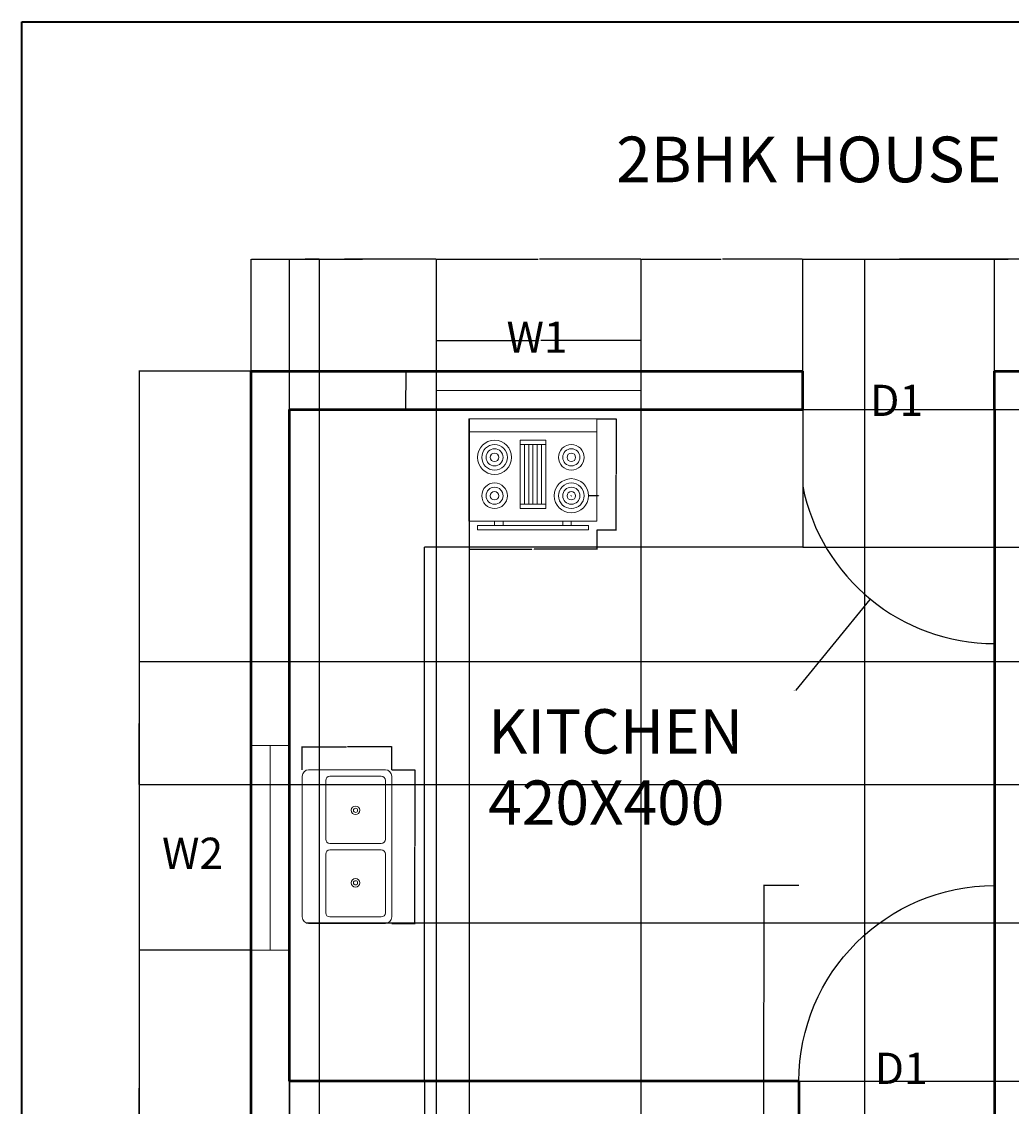
# Model space of a CAD drawing. Units: centimetres. Extents: x 2050 to 3144, y 831 to 2296.
# Tile 6 of 7: x 2050 to 2640, y 1650 to 2296. Entities that reach past the tile are written whole.
import ezdxf

# ---------------------------------------------------------------- set-up
doc = ezdxf.new("R2010")
doc.units = ezdxf.units.CM
for name, color, linetype, lineweight in [('A-ANNO-DIMS', 2, 'Continuous', 18), ('A-ANNO-TEXT', 7, 'Continuous', 18), ('A-ANNO-TTLB', 7, 'Continuous', 35), ('A-AREA-IDEN', 7, 'Continuous', 25), ('A-DOOR', 3, 'Continuous', 25), ('A-EQPM', 9, 'Continuous', 18), ('A-FLOR-CASE', 8, 'Continuous', 25), ('A-FLOR-FIXT', 8, 'Continuous', 18), ('A-GLAZ', 4, 'Continuous', 18), ('A-WALL', 7, 'Continuous', 50)]:
    doc.layers.add(name, color=color, linetype=linetype, lineweight=lineweight)
doc.styles.get("Standard").update_dxf_attribs({"font": 'arial.ttf'})
doc.dimstyles.get("Standard").update_dxf_attribs({"dimtxt": 0.18, "dimasz": 0.18, "dimexe": 0.18, "dimexo": 0.0625, "dimgap": 0.09, "dimtad": 0, "dimtih": 1, "dimtoh": 1, "dimdec": 4, "dimzin": 0, "dimdsep": 46, "dimtxsty": 'Standard', "dimcen": 0.09, "dimadec": 0, "dimazin": 0, "dimtfac": 1, "dimtdec": 4, "dimtofl": 0, "dimtmove": 0, "dimatfit": 3, "dimfxl": 1, "dimtolj": 1, "dimtzin": 0, "dimarcsym": 0})

# ---------------------------------------------------------------- blocks, each defined once
blk = doc.blocks.new('Sink-double - 36 in top')
for p, q in [((-18, -4), (18, -4)), ((-0.75, -18.5), (-0.75, -6.5)), ((0.75, -6.5), (0.75, -18.5))]:
    blk.add_line(p, q)
for points in [[(-16.5, 0), (16.5, 0)], [(-18, -19.5), (-18, -1.5)], [(18, -1.5), (18, -19.5)], [(-16.5, -18.5), (-16.5, -6.5)], [(-15.5, -5.5), (-1.75, -5.5)], [(1.75, -5.5), (15.5, -5.5)], [(16.5, -6.5), (16.5, -18.5)], [(-1.75, -19.5), (-15.5, -19.5)], [(15.5, -19.5), (1.75, -19.5)], [(16.5, -21), (-16.5, -21)]]:
    blk.add_lwpolyline(points)
for centre, radius in [((-8.5, -12.5), 1), ((-8.5, -12.5), 0.5), ((8.5, -12.5), 1), ((8.5, -12.5), 0.5)]:
    blk.add_circle(centre, radius)
for centre, radius, start, end in [((-16.5, -1.5), 1.5, 90, 180), ((16.5, -1.5), 1.5, 0, 90), ((-15.5, -6.5), 1, 90, 180), ((-1.75, -6.5), 1, 0, 90), ((1.75, -6.5), 1, 90, 180), ((15.5, -6.5), 1, 0, 90), ((-16.5, -19.5), 1.5, 180, 270), ((-15.5, -18.5), 1, 180, 270), ((-1.75, -18.5), 1, 270, 0), ((1.75, -18.5), 1, 180, 270), ((15.5, -18.5), 1, 270, 0), ((16.5, -19.5), 1.5, 270, 0)]:
    blk.add_arc(centre, radius, start, end)
blk = doc.blocks.new('Range-Oven - 30 in top')
for p, q in [((0, -3), (30, -3)), ((12, -6), (18, -6)), ((13, -20), (13, -6)), ((14, -6), (14, -20)), ((15, -20), (15, -6)), ((16, -6), (16, -20)), ((17, -20), (17, -6)), ((18, -20), (12, -20)), ((6, -24), (6, -25)), ((8, -25), (8, -24)), ((22, -25), (22, -24)), ((24, -24), (24, -25))]:
    blk.add_line(p, q)
for points in [[(0, -24), (0, 0), (30, 0), (30, -24)], [(12, -21), (12, -5), (18, -5), (18, -21)], [(2, -26), (2, -25), (28, -25), (28, -26)]]:
    blk.add_lwpolyline(points, close=True)
for centre, radius in [((6, -9), 4), ((6, -9), 3), ((6, -9), 2), ((24, -9), 3), ((24, -9), 2), ((6, -9), 1), ((24, -9), 1), ((6, -18), 3), ((24, -18), 4), ((24, -18), 3), ((6, -18), 2), ((6, -18), 1), ((24, -18), 2), ((24, -18), 1)]:
    blk.add_circle(centre, radius)
blk = doc.blocks.new('DOOR-D1-1165')
blk.add_line((116.51, 0), (116.51, 139.37))
blk.add_arc((116.51, 116.51), 116.51, 180, 270)
blk = doc.blocks.new('WIN-1219')
for p, q in [((0, 22.86), (0, 0)), ((121.92, 22.86), (121.92, 0)), ((0, 11.43), (121.92, 11.43))]:
    blk.add_line(p, q)
blk = doc.blocks.new('*D15')
at = {"layer": 'A-ANNO-DIMS', "color": 0, "lineweight": -2, "transparency": 16777216}
for p, q in [((2513.3, 1781.4), (2492.28, 1781.4)), ((2492.46, 1781.22), (2492.46, 1711.9)), ((2492.46, 1642.21), (2492.46, 1711.53)), ((2513.3, 1642.03), (2492.28, 1642.03))]:
    blk.add_line(p, q, dxfattribs=at)
at = {"layer": 'A-ANNO-DIMS', "color": 0, "transparency": 16777216}
for points in [[(2492.43, 1781.22), (2492.49, 1781.22), (2492.46, 1781.4)], [(2492.43, 1642.21), (2492.49, 1642.21), (2492.46, 1642.03)]]:
    blk.add_solid(points, dxfattribs=at)
at = {"layer": 'Defpoints', "color": 0, "transparency": 16777216}
for p in [(2513.36, 1781.4), (2492.46, 1642.03), (2513.36, 1642.03)]:
    blk.add_point(p, dxfattribs=at)
at = {"layer": 'A-ANNO-DIMS', "color": 0, "transparency": 16777216, "insert": (2492.46, 1711.72), "char_height": 0.18, "attachment_point": 5}
blk.add_mtext('\\A1;DOOR D1 139 TYP.', dxfattribs=at)
blk = doc.blocks.new('*D17')
at = {"layer": 'A-ANNO-DIMS', "color": 0, "lineweight": -2, "transparency": 16777216}
for p, q in [((2297.47, 2087.82), (2297.47, 2106.22)), ((2297.65, 2106.04), (2357.25, 2106.04)), ((2419.21, 2106.04), (2359.62, 2106.04)), ((2419.39, 2087.82), (2419.39, 2106.22))]:
    blk.add_line(p, q, dxfattribs=at)
at = {"layer": 'A-ANNO-DIMS', "color": 0, "transparency": 16777216}
for points in [[(2297.65, 2106.07), (2297.65, 2106.01), (2297.47, 2106.04)], [(2419.21, 2106.07), (2419.21, 2106.01), (2419.39, 2106.04)]]:
    blk.add_solid(points, dxfattribs=at)
at = {"layer": 'Defpoints', "color": 0, "transparency": 16777216}
for p in [(2419.39, 2106.04), (2297.47, 2087.75), (2419.39, 2087.75)]:
    blk.add_point(p, dxfattribs=at)
at = {"layer": 'A-ANNO-DIMS', "color": 0, "transparency": 16777216, "insert": (2358.43, 2106.04), "char_height": 0.18, "attachment_point": 5}
blk.add_mtext('\\A1;WINDOW 122 TYP.', dxfattribs=at)
blk = doc.blocks.new('*D18')
at = {"layer": 'A-ANNO-DIMS', "color": 0, "lineweight": -2, "transparency": 16777216}
for p, q in [((2297.41, 2087.75), (2279.01, 2087.75)), ((2279.19, 2087.57), (2279.19, 2076.51)), ((2279.19, 2065.07), (2279.19, 2076.14)), ((2297.41, 2064.89), (2279.01, 2064.89))]:
    blk.add_line(p, q, dxfattribs=at)
at = {"layer": 'A-ANNO-DIMS', "color": 0, "transparency": 16777216}
for points in [[(2279.16, 2087.57), (2279.22, 2087.57), (2279.19, 2087.75)], [(2279.16, 2065.07), (2279.22, 2065.07), (2279.19, 2064.89)]]:
    blk.add_solid(points, dxfattribs=at)
at = {"layer": 'Defpoints', "color": 0, "transparency": 16777216}
for p in [(2279.19, 2087.75), (2297.47, 2087.75), (2297.47, 2064.89)]:
    blk.add_point(p, dxfattribs=at)
at = {"layer": 'A-ANNO-DIMS', "color": 0, "transparency": 16777216, "insert": (2279.19, 2076.32), "char_height": 0.18, "attachment_point": 5}
blk.add_mtext('\\A1;23 TYP.', dxfattribs=at)
blk = doc.blocks.new('*D25')
at = {"layer": 'A-ANNO-DIMS', "color": 0, "lineweight": -2, "transparency": 16777216}
for p, q in [((2270.89, 1850.36), (2284.72, 1850.36)), ((2284.54, 1850.18), (2284.54, 1804.83)), ((2284.54, 1759.1), (2284.54, 1804.46)), ((2270.89, 1758.92), (2284.72, 1758.92))]:
    blk.add_line(p, q, dxfattribs=at)
at = {"layer": 'A-ANNO-DIMS', "color": 0, "transparency": 16777216}
for points in [[(2284.51, 1850.18), (2284.57, 1850.18), (2284.54, 1850.36)], [(2284.51, 1759.1), (2284.57, 1759.1), (2284.54, 1758.92)]]:
    blk.add_solid(points, dxfattribs=at)
at = {"layer": 'Defpoints', "color": 0, "transparency": 16777216}
for p in [(2270.83, 1850.36), (2284.54, 1850.36), (2270.83, 1758.92)]:
    blk.add_point(p, dxfattribs=at)
at = {"layer": 'A-ANNO-DIMS', "color": 0, "transparency": 16777216, "insert": (2284.54, 1804.64), "char_height": 0.18, "attachment_point": 5}
blk.add_mtext('\\A1;SINK 91', dxfattribs=at)
blk = doc.blocks.new('*D26')
at = {"layer": 'A-ANNO-DIMS', "color": 0, "lineweight": -2, "transparency": 16777216}
for p, q in [((2217.49, 1850.42), (2217.49, 1864.26)), ((2217.67, 1864.08), (2243.94, 1864.08)), ((2270.65, 1864.08), (2244.38, 1864.08)), ((2270.83, 1850.42), (2270.83, 1864.26))]:
    blk.add_line(p, q, dxfattribs=at)
at = {"layer": 'A-ANNO-DIMS', "color": 0, "transparency": 16777216}
for points in [[(2217.67, 1864.11), (2217.67, 1864.05), (2217.49, 1864.08)], [(2270.65, 1864.11), (2270.65, 1864.05), (2270.83, 1864.08)]]:
    blk.add_solid(points, dxfattribs=at)
at = {"layer": 'Defpoints', "color": 0, "transparency": 16777216}
for p in [(2217.49, 1864.08), (2217.49, 1850.36), (2270.83, 1850.36)]:
    blk.add_point(p, dxfattribs=at)
at = {"layer": 'A-ANNO-DIMS', "color": 0, "transparency": 16777216, "insert": (2244.16, 1864.08), "char_height": 0.18, "attachment_point": 5}
blk.add_mtext('\\A1;53', dxfattribs=at)
blk = doc.blocks.new('*D27')
at = {"layer": 'A-ANNO-DIMS', "color": 0, "lineweight": -2, "transparency": 16777216}
for p, q in [((2316.84, 1993.19), (2316.84, 1981.64)), ((2393.04, 1993.19), (2393.04, 1981.64)), ((2317.02, 1981.82), (2354.24, 1981.82)), ((2392.86, 1981.82), (2355.63, 1981.82))]:
    blk.add_line(p, q, dxfattribs=at)
at = {"layer": 'A-ANNO-DIMS', "color": 0, "transparency": 16777216}
for points in [[(2317.02, 1981.85), (2317.02, 1981.79), (2316.84, 1981.82)], [(2392.86, 1981.85), (2392.86, 1981.79), (2393.04, 1981.82)]]:
    blk.add_solid(points, dxfattribs=at)
at = {"layer": 'Defpoints', "color": 0, "transparency": 16777216}
for p in [(2316.84, 1993.25), (2393.04, 1993.25), (2393.04, 1981.82)]:
    blk.add_point(p, dxfattribs=at)
at = {"layer": 'A-ANNO-DIMS', "color": 0, "transparency": 16777216, "insert": (2354.94, 1981.82), "char_height": 0.18, "attachment_point": 5}
blk.add_mtext('\\A1;RANGE 76', dxfattribs=at)
blk = doc.blocks.new('*D28')
at = {"layer": 'A-ANNO-DIMS', "color": 0, "lineweight": -2, "transparency": 16777216}
for p, q in [((2393.1, 2059.29), (2404.65, 2059.29)), ((2404.47, 2059.11), (2404.47, 2026.45)), ((2404.47, 1993.43), (2404.47, 2026.09)), ((2393.1, 1993.25), (2404.65, 1993.25))]:
    blk.add_line(p, q, dxfattribs=at)
at = {"layer": 'A-ANNO-DIMS', "color": 0, "transparency": 16777216}
for points in [[(2404.44, 2059.11), (2404.5, 2059.11), (2404.47, 2059.29)], [(2404.44, 1993.43), (2404.5, 1993.43), (2404.47, 1993.25)]]:
    blk.add_solid(points, dxfattribs=at)
at = {"layer": 'Defpoints', "color": 0, "transparency": 16777216}
for p in [(2393.04, 2059.29), (2404.47, 2059.29), (2393.04, 1993.25)]:
    blk.add_point(p, dxfattribs=at)
at = {"layer": 'A-ANNO-DIMS', "color": 0, "transparency": 16777216, "insert": (2404.47, 2026.27), "char_height": 0.18, "attachment_point": 5}
blk.add_mtext('\\A1;66', dxfattribs=at)
blk = doc.blocks.new('*D32')
at = {"layer": 'A-ANNO-DIMS', "color": 0, "lineweight": -2, "transparency": 16777216}
for p, q in [((2186.94, 2087.75), (2120.23, 2087.75)), ((2120.41, 2087.57), (2120.41, 1582.22)), ((2120.41, 1076.49), (2120.41, 1581.85)), ((2186.94, 1076.31), (2120.23, 1076.31))]:
    blk.add_line(p, q, dxfattribs=at)
at = {"layer": 'A-ANNO-DIMS', "color": 0, "transparency": 16777216}
for points in [[(2120.38, 2087.57), (2120.44, 2087.57), (2120.41, 2087.75)], [(2120.38, 1076.49), (2120.44, 1076.49), (2120.41, 1076.31)]]:
    blk.add_solid(points, dxfattribs=at)
at = {"layer": 'Defpoints', "color": 0, "transparency": 16777216}
for p in [(2120.41, 2087.75), (2187.01, 2087.75), (2187.01, 1076.31)]:
    blk.add_point(p, dxfattribs=at)
at = {"layer": 'A-ANNO-DIMS', "color": 0, "transparency": 16777216, "insert": (2120.41, 1582.03), "char_height": 0.18, "attachment_point": 5}
blk.add_mtext('\\A1;1011.4', dxfattribs=at)
blk = doc.blocks.new('*D33')
at = {"layer": 'A-ANNO-DIMS', "color": 0, "lineweight": -2, "transparency": 16777216}
for p, q in [((2187.01, 2087.82), (2187.01, 2154.53)), ((2187.19, 2154.35), (2241.78, 2154.35)), ((2297.29, 2154.35), (2242.7, 2154.35)), ((2297.47, 2087.82), (2297.47, 2154.53))]:
    blk.add_line(p, q, dxfattribs=at)
at = {"layer": 'A-ANNO-DIMS', "color": 0, "transparency": 16777216}
for points in [[(2187.19, 2154.38), (2187.19, 2154.32), (2187.01, 2154.35)], [(2297.29, 2154.38), (2297.29, 2154.32), (2297.47, 2154.35)]]:
    blk.add_solid(points, dxfattribs=at)
at = {"layer": 'Defpoints', "color": 0, "transparency": 16777216}
for p in [(2297.47, 2154.35), (2187.01, 2087.75), (2297.47, 2087.75)]:
    blk.add_point(p, dxfattribs=at)
at = {"layer": 'A-ANNO-DIMS', "color": 0, "transparency": 16777216, "insert": (2242.24, 2154.35), "char_height": 0.18, "attachment_point": 5}
blk.add_mtext('\\A1;110.47', dxfattribs=at)
blk = doc.blocks.new('*D34')
at = {"layer": 'A-ANNO-DIMS', "color": 0, "lineweight": -2, "transparency": 16777216}
for p, q in [((2419.39, 2087.82), (2419.39, 2154.53)), ((2419.57, 2154.35), (2467.12, 2154.35)), ((2515.45, 2154.35), (2467.9, 2154.35)), ((2515.63, 2087.82), (2515.63, 2154.53))]:
    blk.add_line(p, q, dxfattribs=at)
at = {"layer": 'A-ANNO-DIMS', "color": 0, "transparency": 16777216}
for points in [[(2419.57, 2154.38), (2419.57, 2154.32), (2419.39, 2154.35)], [(2515.45, 2154.38), (2515.45, 2154.32), (2515.63, 2154.35)]]:
    blk.add_solid(points, dxfattribs=at)
at = {"layer": 'Defpoints', "color": 0, "transparency": 16777216}
for p in [(2515.63, 2154.35), (2419.39, 2087.75), (2515.63, 2087.75)]:
    blk.add_point(p, dxfattribs=at)
at = {"layer": 'A-ANNO-DIMS', "color": 0, "transparency": 16777216, "insert": (2467.51, 2154.35), "char_height": 0.18, "attachment_point": 5}
blk.add_mtext('\\A1;96.23', dxfattribs=at)
blk = doc.blocks.new('*D35')
at = {"layer": 'A-ANNO-DIMS', "color": 0, "lineweight": -2, "transparency": 16777216}
for p, q in [((2515.63, 2087.82), (2515.63, 2154.53)), ((2515.81, 2154.35), (2572.29, 2154.35)), ((2629.69, 2154.35), (2573.2, 2154.35)), ((2629.87, 2087.82), (2629.87, 2154.53))]:
    blk.add_line(p, q, dxfattribs=at)
at = {"layer": 'A-ANNO-DIMS', "color": 0, "transparency": 16777216}
for points in [[(2515.81, 2154.38), (2515.81, 2154.32), (2515.63, 2154.35)], [(2629.69, 2154.38), (2629.69, 2154.32), (2629.87, 2154.35)]]:
    blk.add_solid(points, dxfattribs=at)
at = {"layer": 'Defpoints', "color": 0, "transparency": 16777216}
for p in [(2629.87, 2154.35), (2515.63, 2087.75), (2629.87, 2087.75)]:
    blk.add_point(p, dxfattribs=at)
at = {"layer": 'A-ANNO-DIMS', "color": 0, "transparency": 16777216, "insert": (2572.75, 2154.35), "char_height": 0.18, "attachment_point": 5}
blk.add_mtext('\\A1;114.24', dxfattribs=at)
blk = doc.blocks.new('*D42')
at = {"layer": 'A-ANNO-DIMS', "color": 0, "lineweight": -2, "transparency": 16777216}
for p, q in [((2186.94, 1742.97), (2120.23, 1742.97)), ((2120.41, 1742.79), (2120.41, 1661.12)), ((2120.41, 1579.07), (2120.41, 1660.75)), ((2186.94, 1578.89), (2120.23, 1578.89))]:
    blk.add_line(p, q, dxfattribs=at)
at = {"layer": 'A-ANNO-DIMS', "color": 0, "transparency": 16777216}
for points in [[(2120.38, 1742.79), (2120.44, 1742.79), (2120.41, 1742.97)], [(2120.38, 1579.07), (2120.44, 1579.07), (2120.41, 1578.89)]]:
    blk.add_solid(points, dxfattribs=at)
at = {"layer": 'Defpoints', "color": 0, "transparency": 16777216}
for p in [(2120.41, 1742.97), (2187.01, 1742.97), (2187.01, 1578.89)]:
    blk.add_point(p, dxfattribs=at)
at = {"layer": 'A-ANNO-DIMS', "color": 0, "transparency": 16777216, "insert": (2120.41, 1660.93), "char_height": 0.18, "attachment_point": 5}
blk.add_mtext('\\A1;164.08', dxfattribs=at)
blk = doc.blocks.new('*D47')
at = {"layer": 'A-ANNO-DIMS', "color": 0, "lineweight": -2, "transparency": 16777216}
for p, q in [((2209.87, 1099.24), (2209.87, 2154.53)), ((2210.05, 2154.35), (2253.35, 2154.35)), ((2297.29, 2154.35), (2253.99, 2154.35)), ((2297.47, 1099.24), (2297.47, 2154.53))]:
    blk.add_line(p, q, dxfattribs=at)
at = {"layer": 'A-ANNO-DIMS', "color": 0, "transparency": 16777216}
for points in [[(2210.05, 2154.38), (2210.05, 2154.32), (2209.87, 2154.35)], [(2297.29, 2154.38), (2297.29, 2154.32), (2297.47, 2154.35)]]:
    blk.add_solid(points, dxfattribs=at)
at = {"layer": 'Defpoints', "color": 0, "transparency": 16777216}
for p in [(2297.47, 2154.35), (2209.87, 1099.17), (2297.47, 1099.17)]:
    blk.add_point(p, dxfattribs=at)
at = {"layer": 'A-ANNO-DIMS', "color": 0, "transparency": 16777216, "insert": (2253.67, 2154.35), "char_height": 0.18, "attachment_point": 5}
blk.add_mtext('\\A1;87.6', dxfattribs=at)
blk = doc.blocks.new('*D48')
at = {"layer": 'A-ANNO-DIMS', "color": 0, "lineweight": -2, "transparency": 16777216}
for p, q in [((2552.73, 1211.94), (2552.73, 2154.53)), ((2552.91, 2154.35), (2610.59, 2154.35)), ((2669.05, 2154.35), (2611.37, 2154.35)), ((2669.23, 1211.94), (2669.23, 2154.53))]:
    blk.add_line(p, q, dxfattribs=at)
at = {"layer": 'A-ANNO-DIMS', "color": 0, "transparency": 16777216}
for points in [[(2552.91, 2154.38), (2552.91, 2154.32), (2552.73, 2154.35)], [(2669.05, 2154.38), (2669.05, 2154.32), (2669.23, 2154.35)]]:
    blk.add_solid(points, dxfattribs=at)
at = {"layer": 'Defpoints', "color": 0, "transparency": 16777216}
for p in [(2669.23, 2154.35), (2552.73, 1211.87), (2669.23, 1211.87)]:
    blk.add_point(p, dxfattribs=at)
at = {"layer": 'A-ANNO-DIMS', "color": 0, "transparency": 16777216, "insert": (2610.98, 2154.35), "char_height": 0.18, "attachment_point": 5}
blk.add_mtext('\\A1;116.5', dxfattribs=at)
blk = doc.blocks.new('*D53')
at = {"layer": 'A-ANNO-DIMS', "color": 0, "lineweight": -2, "transparency": 16777216}
for p, q in [((2209.87, 1664.83), (2209.87, 1009.53)), ((2290.25, 1664.83), (2290.25, 1009.53)), ((2210.05, 1009.71), (2249.67, 1009.71)), ((2290.07, 1009.71), (2250.45, 1009.71))]:
    blk.add_line(p, q, dxfattribs=at)
at = {"layer": 'A-ANNO-DIMS', "color": 0, "transparency": 16777216}
for points in [[(2210.05, 1009.74), (2210.05, 1009.68), (2209.87, 1009.71)], [(2290.07, 1009.74), (2290.07, 1009.68), (2290.25, 1009.71)]]:
    blk.add_solid(points, dxfattribs=at)
at = {"layer": 'Defpoints', "color": 0, "transparency": 16777216}
for p in [(2209.87, 1664.89), (2290.25, 1664.89), (2290.25, 1009.71)]:
    blk.add_point(p, dxfattribs=at)
at = {"layer": 'A-ANNO-DIMS', "color": 0, "transparency": 16777216, "insert": (2250.06, 1009.71), "char_height": 0.18, "attachment_point": 5}
blk.add_mtext('\\A1;80.39', dxfattribs=at)
blk = doc.blocks.new('*D54')
at = {"layer": 'A-ANNO-DIMS', "color": 0, "lineweight": -2, "transparency": 16777216}
for p, q in [((2515.69, 2064.89), (3042.37, 2064.89)), ((3042.19, 2064.71), (3042.19, 2024.09)), ((3042.19, 1983.1), (3042.19, 2023.73)), ((2515.69, 1982.92), (3042.37, 1982.92))]:
    blk.add_line(p, q, dxfattribs=at)
at = {"layer": 'A-ANNO-DIMS', "color": 0, "transparency": 16777216}
for points in [[(3042.16, 2064.71), (3042.22, 2064.71), (3042.19, 2064.89)], [(3042.16, 1983.1), (3042.22, 1983.1), (3042.19, 1982.92)]]:
    blk.add_solid(points, dxfattribs=at)
at = {"layer": 'Defpoints', "color": 0, "transparency": 16777216}
for p in [(2515.63, 2064.89), (3042.19, 2064.89), (2515.63, 1982.92)]:
    blk.add_point(p, dxfattribs=at)
at = {"layer": 'A-ANNO-DIMS', "color": 0, "transparency": 16777216, "insert": (3042.19, 2023.91), "char_height": 0.18, "attachment_point": 5}
blk.add_mtext('\\A1;81.97', dxfattribs=at)
blk = doc.blocks.new('*D61')
at = {"layer": 'A-ANNO-DIMS', "color": 0, "lineweight": -2, "transparency": 16777216}
for p, q in [((2552.73, 1328.44), (2552.73, 2154.53)), ((2552.91, 2154.35), (2638.04, 2154.35)), ((2723.95, 2154.35), (2638.81, 2154.35)), ((2724.13, 1334.5), (2724.13, 2154.53))]:
    blk.add_line(p, q, dxfattribs=at)
at = {"layer": 'A-ANNO-DIMS', "color": 0, "transparency": 16777216}
for points in [[(2552.91, 2154.38), (2552.91, 2154.32), (2552.73, 2154.35)], [(2723.95, 2154.38), (2723.95, 2154.32), (2724.13, 2154.35)]]:
    blk.add_solid(points, dxfattribs=at)
at = {"layer": 'Defpoints', "color": 0, "transparency": 16777216}
for p in [(2724.13, 2154.35), (2724.13, 1334.43), (2552.73, 1328.38)]:
    blk.add_point(p, dxfattribs=at)
at = {"layer": 'A-ANNO-DIMS', "color": 0, "transparency": 16777216, "insert": (2638.43, 2154.35), "char_height": 0.18, "attachment_point": 5}
blk.add_mtext('\\A1;171.4', dxfattribs=at)
blk = doc.blocks.new('*D63')
at = {"layer": 'A-ANNO-DIMS', "color": 0, "lineweight": -2, "transparency": 16777216}
for p, q in [((2297.47, 1099.24), (2297.47, 2154.53)), ((2297.65, 2154.35), (2357.98, 2154.35)), ((2419.21, 2154.35), (2358.89, 2154.35)), ((2419.39, 1099.24), (2419.39, 2154.53))]:
    blk.add_line(p, q, dxfattribs=at)
at = {"layer": 'A-ANNO-DIMS', "color": 0, "transparency": 16777216}
for points in [[(2297.65, 2154.38), (2297.65, 2154.32), (2297.47, 2154.35)], [(2419.21, 2154.38), (2419.21, 2154.32), (2419.39, 2154.35)]]:
    blk.add_solid(points, dxfattribs=at)
at = {"layer": 'Defpoints', "color": 0, "transparency": 16777216}
for p in [(2419.39, 2154.35), (2297.47, 1099.17), (2419.39, 1099.17)]:
    blk.add_point(p, dxfattribs=at)
at = {"layer": 'A-ANNO-DIMS', "color": 0, "transparency": 16777216, "insert": (2358.43, 2154.35), "char_height": 0.18, "attachment_point": 5}
blk.add_mtext('\\A1;121.92', dxfattribs=at)
blk = doc.blocks.new('*D66')
at = {"layer": 'A-ANNO-DIMS', "color": 0, "lineweight": -2, "transparency": 16777216}
for p, q in [((2209.87, 1139.14), (2209.87, 2154.53)), ((2210.05, 2154.35), (2218.38, 2154.35)), ((2227.62, 2154.35), (2219.29, 2154.35)), ((2227.8, 1152.03), (2227.8, 2154.53))]:
    blk.add_line(p, q, dxfattribs=at)
at = {"layer": 'A-ANNO-DIMS', "color": 0, "transparency": 16777216}
for points in [[(2210.05, 2154.38), (2210.05, 2154.32), (2209.87, 2154.35)], [(2227.62, 2154.38), (2227.62, 2154.32), (2227.8, 2154.35)]]:
    blk.add_solid(points, dxfattribs=at)
at = {"layer": 'Defpoints', "color": 0, "transparency": 16777216}
for p in [(2227.8, 2154.35), (2227.8, 1151.97), (2209.87, 1139.08)]:
    blk.add_point(p, dxfattribs=at)
at = {"layer": 'A-ANNO-DIMS', "color": 0, "transparency": 16777216, "insert": (2218.83, 2154.35), "char_height": 0.18, "attachment_point": 5}
blk.add_mtext('\\A1;17.933', dxfattribs=at)
blk = doc.blocks.new('*D69')
at = {"layer": 'A-ANNO-DIMS', "color": 0, "lineweight": -2, "transparency": 16777216}
for p, q in [((2822.82, 1914.73), (2120.23, 1914.73)), ((2120.41, 1914.55), (2120.41, 1878.23)), ((2120.41, 1841.54), (2120.41, 1877.86)), ((2933.72, 1841.36), (2120.23, 1841.36))]:
    blk.add_line(p, q, dxfattribs=at)
at = {"layer": 'A-ANNO-DIMS', "color": 0, "transparency": 16777216}
for points in [[(2120.38, 1914.55), (2120.44, 1914.55), (2120.41, 1914.73)], [(2120.38, 1841.54), (2120.44, 1841.54), (2120.41, 1841.36)]]:
    blk.add_solid(points, dxfattribs=at)
at = {"layer": 'Defpoints', "color": 0, "transparency": 16777216}
for p in [(2120.41, 1914.73), (2822.89, 1914.73), (2933.78, 1841.36)]:
    blk.add_point(p, dxfattribs=at)
at = {"layer": 'A-ANNO-DIMS', "color": 0, "transparency": 16777216, "insert": (2120.41, 1878.05), "char_height": 0.18, "attachment_point": 5}
blk.add_mtext('\\A1;73.38', dxfattribs=at)
blk = doc.blocks.new('*D70')
at = {"layer": 'A-ANNO-DIMS', "color": 0, "lineweight": -2, "transparency": 16777216}
for p, q in [((2209.87, 2064.83), (2209.87, 1009.53)), ((2316.84, 2059.23), (2316.84, 1009.53)), ((2210.05, 1009.71), (2262.9, 1009.71)), ((2316.66, 1009.71), (2263.81, 1009.71))]:
    blk.add_line(p, q, dxfattribs=at)
at = {"layer": 'A-ANNO-DIMS', "color": 0, "transparency": 16777216}
for points in [[(2210.05, 1009.74), (2210.05, 1009.68), (2209.87, 1009.71)], [(2316.66, 1009.74), (2316.66, 1009.68), (2316.84, 1009.71)]]:
    blk.add_solid(points, dxfattribs=at)
at = {"layer": 'Defpoints', "color": 0, "transparency": 16777216}
for p in [(2209.87, 2064.89), (2316.84, 2059.29), (2316.84, 1009.71)]:
    blk.add_point(p, dxfattribs=at)
at = {"layer": 'A-ANNO-DIMS', "color": 0, "transparency": 16777216, "insert": (2263.35, 1009.71), "char_height": 0.18, "attachment_point": 5}
blk.add_mtext('\\A1;106.97', dxfattribs=at)
blk = doc.blocks.new('*D71')
at = {"layer": 'A-ANNO-DIMS', "color": 0, "lineweight": -2, "transparency": 16777216}
for p, q in [((2219.88, 1759.22), (3042.37, 1759.22)), ((3042.19, 1759.04), (3042.19, 1712.24)), ((3042.19, 1665.07), (3042.19, 1711.88)), ((2209.93, 1664.89), (3042.37, 1664.89))]:
    blk.add_line(p, q, dxfattribs=at)
at = {"layer": 'A-ANNO-DIMS', "color": 0, "transparency": 16777216}
for points in [[(3042.16, 1759.04), (3042.22, 1759.04), (3042.19, 1759.22)], [(3042.16, 1665.07), (3042.22, 1665.07), (3042.19, 1664.89)]]:
    blk.add_solid(points, dxfattribs=at)
at = {"layer": 'Defpoints', "color": 0, "transparency": 16777216}
for p in [(2219.81, 1759.22), (3042.19, 1759.22), (2209.87, 1664.89)]:
    blk.add_point(p, dxfattribs=at)
at = {"layer": 'A-ANNO-DIMS', "color": 0, "transparency": 16777216, "insert": (3042.19, 1712.06), "char_height": 0.18, "attachment_point": 5}
blk.add_mtext('\\A1;94.33', dxfattribs=at)
blk = doc.blocks.new('*D75')
at = {"layer": 'A-ANNO-DIMS', "color": 0, "lineweight": -2, "transparency": 16777216}
for p, q in [((2629.78, 2042.03), (2629.96, 2042.03)), ((2629.87, 2041.94), (2629.87, 2042.12)), ((2511.69, 1897.87), (2555.89, 1951.79)), ((2511.51, 1897.87), (2511.69, 1897.87))]:
    blk.add_line(p, q, dxfattribs=at)
at = {"layer": 'A-ANNO-DIMS', "color": 0, "transparency": 16777216}
blk.add_solid([(2555.87, 1951.81), (2555.92, 1951.77), (2556.01, 1951.93)], dxfattribs=at)
at = {"layer": 'Defpoints', "color": 0, "transparency": 16777216}
for p in [(2629.87, 2042.03), (2556.01, 1951.93)]:
    blk.add_point(p, dxfattribs=at)
at = {"layer": 'A-ANNO-DIMS', "color": 0, "transparency": 16777216, "insert": (2510.84, 1897.87), "char_height": 0.18, "attachment_point": 5}
blk.add_mtext('\\A1;5X R116.5', dxfattribs=at)
blk = doc.blocks.new('*D81')
at = {"layer": 'A-ANNO-DIMS', "color": 0, "lineweight": -2, "transparency": 16777216}
for p, q in [((2377.71, 2013.57), (2377.89, 2013.57)), ((2377.8, 2013.48), (2377.8, 2013.66)), ((2394.05, 2013.57), (2388.14, 2013.57))]:
    blk.add_line(p, q, dxfattribs=at)
at = {"layer": 'A-ANNO-DIMS', "color": 0, "transparency": 16777216}
blk.add_solid([(2388.14, 2013.6), (2388.14, 2013.54), (2387.96, 2013.57)], dxfattribs=at)
at = {"layer": 'Defpoints', "color": 0, "transparency": 16777216}
for p in [(2367.64, 2013.57), (2387.96, 2013.57)]:
    blk.add_point(p, dxfattribs=at)
at = {"layer": 'A-ANNO-DIMS', "color": 0, "transparency": 16777216, "insert": (2394.73, 2013.57), "char_height": 0.18, "attachment_point": 5}
blk.add_mtext('\\A1;2X ∅20.32', dxfattribs=at)

msp = doc.modelspace()

# ---------------------------------------------------------------- linework, layer by layer
at = {"layer": 'A-ANNO-TTLB'}
msp.add_lwpolyline([(2050.3641, 2295.8578), (3143.7558, 2295.8578), (3143.7558, 830.6902), (2050.3641, 830.6902)], close=True, dxfattribs=at)
at = {"layer": 'A-DOOR'}
msp.add_line((2629.8665, 1925.5295), (2629.8665, 2064.8948), dxfattribs=at)
msp.add_arc((2629.8665, 2042.0348), 116.5053, 191.3156614, 270, dxfattribs=at)
at = {"layer": 'A-FLOR-CASE'}
for p, q in [((2515.6259, 2064.8948), (2515.6259, 1982.92)), ((2515.6259, 1982.92), (2290.2526, 1982.92)), ((2290.2526, 1664.8948), (2290.2526, 1982.92))]:
    msp.add_line(p, q, dxfattribs=at)
at = {"layer": 'A-WALL'}
for p, q in [((2187.0065, 2087.7548), (2515.6259, 2087.7548)), ((2187.0065, 1076.3148), (2187.0065, 2087.7548)), ((2515.6259, 2064.8948), (2515.6259, 2087.7548)), ((2629.8665, 2064.8948), (2629.8665, 2087.7548)), ((2629.8665, 2087.7548), (2975.5865, 2087.7548)), ((2209.8665, 2064.8948), (2515.6259, 2064.8948)), ((2209.8665, 1664.8948), (2209.8665, 2064.8948)), ((2629.8665, 2064.8948), (2629.8665, 1642.0348)), ((2513.3612, 1664.8948), (2209.8665, 1664.8948)), ((2513.3612, 1664.8948), (2513.3612, 1642.0348)), ((2629.8665, 1664.8948), (2629.8665, 1664.8948))]:
    msp.add_line(p, q, dxfattribs=at)

# ---------------------------------------------------------------- block references
at = {"layer": 'A-DOOR', "extrusion": (0, 0, -1), "zscale": -1, "rotation": 180}
msp.add_blockref('DOOR-D1-1165', (-2513.361, 1781.4006), dxfattribs=at)
at = {"layer": 'A-EQPM', "xscale": 2.54, "yscale": 2.54, "zscale": 2.54}
msp.add_blockref('Range-Oven - 30 in top', (2316.8368, 2059.2924), dxfattribs=at)
at = {"layer": 'A-FLOR-FIXT', "xscale": 2.54, "yscale": 2.54, "zscale": 2.54, "rotation": 90}
msp.add_blockref('Sink-double - 36 in top', (2217.4865, 1804.6424), dxfattribs=at)
at = {"layer": 'A-GLAZ'}
msp.add_blockref('WIN-1219', (2297.473, 2064.895), dxfattribs=at)
at = {"layer": 'A-GLAZ', "rotation": 269.9999999999998}
msp.add_blockref('WIN-1219', (2187.0067, 1864.8951), dxfattribs=at)

# ---------------------------------------------------------------- texts
at = {"layer": 'A-ANNO-TEXT'}
for s, p in [('W1', (2339.1988, 2098.6729)), ('D1', (2555.799, 2061.0524)), ('W2', (2133.9768, 1791.3392)), ('D1', (2558.5383, 1663.3043))]:
    msp.add_text(s, height=18.59595, dxfattribs=at).set_placement(p)
at = {"layer": 'A-ANNO-TTLB'}
msp.add_text('2BHK HOUSE PLAN', height=27.192544, dxfattribs=at).set_placement((2404.4801, 2200.2444))
at = {"layer": 'A-AREA-IDEN'}
for s, p in [('KITCHEN', (2328.3208, 1860.0322)), ('420X400', (2328.3208, 1817.612))]:
    msp.add_text(s, height=26.40684, dxfattribs=at).set_placement(p)

# ---------------------------------------------------------------- dimensions: what is measured, and where the dimension line sits
at = {"layer": 'A-ANNO-DIMS'}
for base, p1, p2, override, picture, middle in [((2297.4733, 2154.3548), (2187.0065, 2087.7548), (2297.4733, 2087.7548), {"dimdec": 2, "dimlfac": 1, "dimrnd": 0, "dimzin": 0, "dimdsep": 46, "dimlunit": 2}, '*D33', (2242.2399, 2154.3548)), ((2297.4733, 2154.3548), (2209.8665, 1099.1748), (2297.4733, 1099.1748), {"dimdec": 1, "dimlfac": 1, "dimrnd": 0, "dimzin": 0, "dimdsep": 46, "dimlunit": 2}, '*D47', (2253.6699, 2154.3548)), ((2227.7996, 2154.3548), (2209.8665, 1139.0811), (2227.7996, 1151.9671), {"dimdec": 3, "dimlfac": 1, "dimrnd": 0, "dimzin": 0, "dimdsep": 46, "dimlunit": 2}, '*D66', (2218.8331, 2154.3548)), ((2419.3933, 2154.3548), (2297.4733, 1099.1748), (2419.3933, 1099.1748), {"dimdec": 2, "dimlfac": 1, "dimrnd": 0, "dimzin": 0, "dimdsep": 46, "dimlunit": 2}, '*D63', (2358.4333, 2154.3548)), ((2515.6259, 2154.3548), (2419.3933, 2087.7548), (2515.6259, 2087.7548), {"dimdec": 2, "dimlfac": 1, "dimrnd": 0, "dimzin": 0, "dimdsep": 46, "dimlunit": 2}, '*D34', (2467.5096, 2154.3548)), ((2629.8665, 2154.3548), (2515.6259, 2087.7548), (2629.8665, 2087.7548), {"dimdec": 2, "dimlfac": 1, "dimrnd": 0, "dimzin": 0, "dimdsep": 46, "dimlunit": 2}, '*D35', (2572.7462, 2154.3548)), ((2669.2319, 2154.3548), (2552.7265, 1211.8748), (2669.2319, 1211.8748), {"dimdec": 1, "dimlfac": 1, "dimrnd": 0, "dimzin": 0, "dimdsep": 46, "dimlunit": 2}, '*D48', (2610.9792, 2154.3548)), ((2724.1318, 2154.3548), (2552.7265, 1328.3801), (2724.1318, 1334.433), {"dimdec": 1, "dimlfac": 1, "dimrnd": 0, "dimzin": 0, "dimdsep": 46, "dimlunit": 2}, '*D61', (2638.4292, 2154.3548)), ((2316.8368, 1009.7148), (2209.8665, 2064.8948), (2316.8368, 2059.2924), {"dimdec": 2, "dimlfac": 1, "dimrnd": 0, "dimzin": 0, "dimdsep": 46, "dimlunit": 2}, '*D70', (2263.3517, 1009.7148)), ((2290.2526, 1009.7148), (2209.8665, 1664.8948), (2290.2526, 1664.8948), {"dimdec": 2, "dimlfac": 1, "dimrnd": 0, "dimzin": 0, "dimdsep": 46, "dimlunit": 2}, '*D53', (2250.0596, 1009.7148))]:
    dim = msp.add_linear_dim(base=base, p1=p1, p2=p2, dimstyle='Standard', override=override, dxfattribs=at)
    dim.commit()
    dim.dimension.update_dxf_attribs({"geometry": picture, "text_midpoint": middle})
for base, p1, p2, text, picture, middle in [((2419.3933, 2106.0428), (2297.4733, 2087.7548), (2419.3933, 2087.7548), 'WINDOW <> TYP.', '*D17', (2358.4333, 2106.0428)), ((2393.0368, 1981.8224), (2316.8368, 1993.2524), (2393.0368, 1993.2524), 'RANGE <>', '*D27', (2354.9368, 1981.8224))]:
    dim = msp.add_linear_dim(base=base, p1=p1, p2=p2, text=text, dimstyle='Standard', override={"dimdec": 0, "dimlfac": 1, "dimrnd": 0, "dimzin": 0, "dimdsep": 46, "dimlunit": 2}, dxfattribs=at)
    dim.commit()
    dim.dimension.update_dxf_attribs({"geometry": picture, "text_midpoint": middle})
for base, p1, p2, angle, override, picture, middle in [((2120.4065, 2087.7548), (2187.0065, 1076.3148), (2187.0065, 2087.7548), 90, {"dimdec": 1, "dimlfac": 1, "dimrnd": 0, "dimzin": 0, "dimdsep": 46, "dimlunit": 2}, '*D32', (2120.4065, 1582.0348)), ((3042.1865, 2064.8948), (2515.6259, 1982.92), (2515.6259, 2064.8948), 90, {"dimdec": 2, "dimlfac": 1, "dimrnd": 0, "dimzin": 0, "dimdsep": 46, "dimlunit": 2}, '*D54', (3042.1865, 2023.9074)), ((2404.4668, 2059.2924), (2393.0368, 1993.2524), (2393.0368, 2059.2924), 90, {"dimdec": 0, "dimlfac": 1, "dimrnd": 0, "dimzin": 0, "dimdsep": 46, "dimlunit": 2}, '*D28', (2404.4668, 2026.2724)), ((2120.4065, 1914.7348), (2933.7791, 1841.3577), (2822.8865, 1914.7348), 90, {"dimdec": 2, "dimlfac": 1, "dimrnd": 0, "dimzin": 0, "dimdsep": 46, "dimlunit": 2}, '*D69', (2120.4065, 1878.0462)), ((2217.4865, 1864.0784), (2270.8265, 1850.3624), (2217.4865, 1850.3624), 180, {"dimdec": 0, "dimlfac": 1, "dimrnd": 0, "dimzin": 0, "dimdsep": 46, "dimlunit": 2}, '*D26', (2244.1565, 1864.0784)), ((3042.1865, 1759.2218), (2209.8665, 1664.8948), (2219.8135, 1759.2218), 90, {"dimdec": 2, "dimlfac": 1, "dimrnd": 0, "dimzin": 0, "dimdsep": 46, "dimlunit": 2}, '*D71', (3042.1865, 1712.0583)), ((2120.4065, 1742.9748), (2187.0065, 1578.8921), (2187.0065, 1742.9748), 90, {"dimdec": 2, "dimlfac": 1, "dimrnd": 0, "dimzin": 0, "dimdsep": 46, "dimlunit": 2}, '*D42', (2120.4065, 1660.9335))]:
    dim = msp.add_linear_dim(base=base, p1=p1, p2=p2, angle=angle, dimstyle='Standard', override=override, dxfattribs=at)
    dim.commit()
    dim.dimension.update_dxf_attribs({"geometry": picture, "text_midpoint": middle})
for base, p1, p2, angle, text, picture, middle in [((2279.1853, 2087.7548), (2297.4733, 2064.8948), (2297.4733, 2087.7548), 90, '<> TYP.', '*D18', (2279.1853, 2076.3248)), ((2284.5425, 1850.3624), (2270.8265, 1758.9224), (2270.8265, 1850.3624), 90, 'SINK <>', '*D25', (2284.5425, 1804.6424)), ((2492.4564, 1642.0348), (2513.3612, 1781.4001), (2513.3612, 1642.0348), 270, 'DOOR D1 <> TYP.', '*D15', (2492.4564, 1711.7175))]:
    dim = msp.add_linear_dim(base=base, p1=p1, p2=p2, angle=angle, text=text, dimstyle='Standard', override={"dimdec": 0, "dimlfac": 1, "dimrnd": 0, "dimzin": 0, "dimdsep": 46, "dimlunit": 2}, dxfattribs=at)
    dim.commit()
    dim.dimension.update_dxf_attribs({"geometry": picture, "text_midpoint": middle})
dim = msp.add_radius_dim(center=(2629.8665, 2042.0348), mpoint=(2556.0078, 1951.9327), text='5X <>', dimstyle='Standard', override={"dimdec": 1, "dimlfac": 1, "dimrnd": 0, "dimzin": 0, "dimdsep": 46, "dimlunit": 2}, dxfattribs=at)
dim.commit()
dim.dimension.update_dxf_attribs({"geometry": '*D75', "text_midpoint": (2510.8386, 1897.8715), "dimtype": 164})
dim = msp.add_diameter_dim_2p(p1=(2367.6368, 2013.5729), p2=(2387.9568, 2013.572), text='2X <>', dimstyle='Standard', override={"dimdec": 2, "dimlfac": 1, "dimrnd": 0, "dimzin": 0, "dimdsep": 46, "dimlunit": 2}, dxfattribs=at)
dim.commit()
dim.dimension.update_dxf_attribs({"geometry": '*D81', "text_midpoint": (2394.0528, 2013.5717), "dimtype": 163})

doc.saveas('drawing.dxf')
